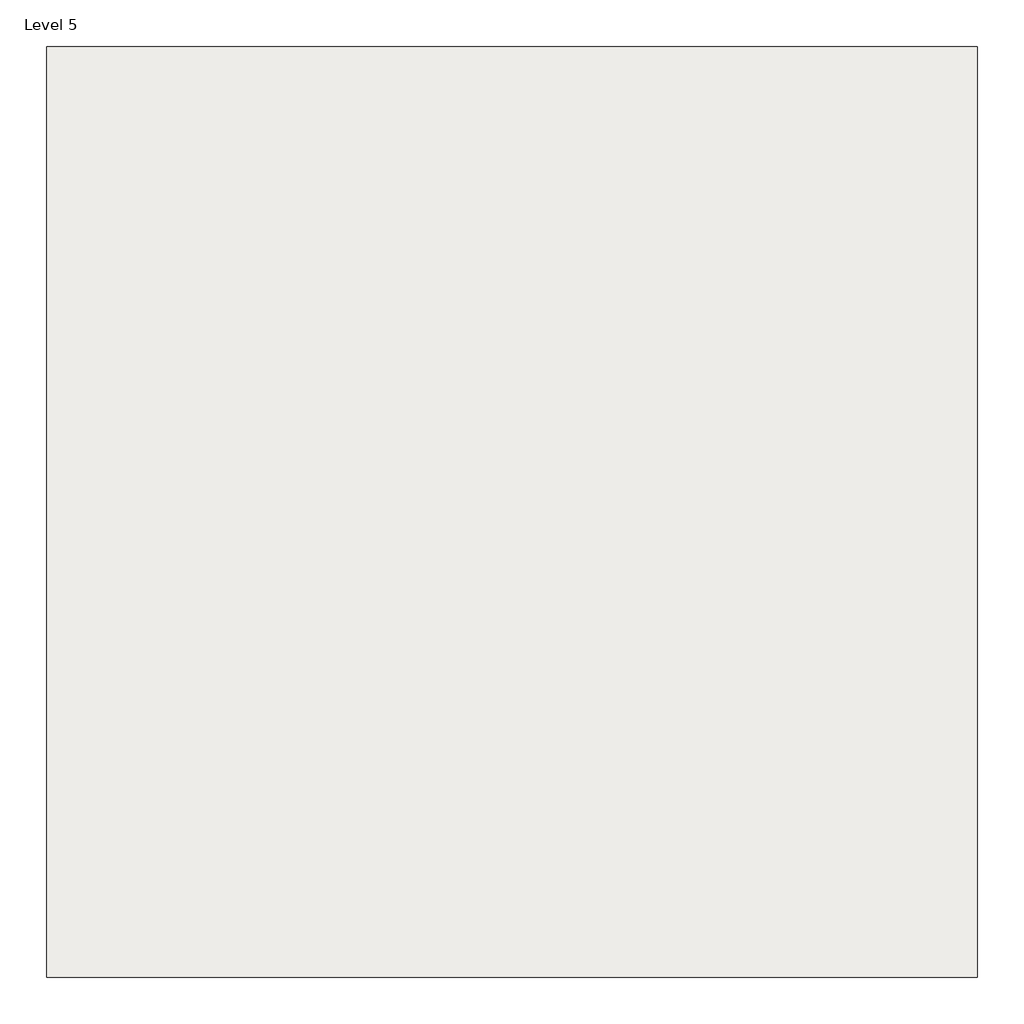
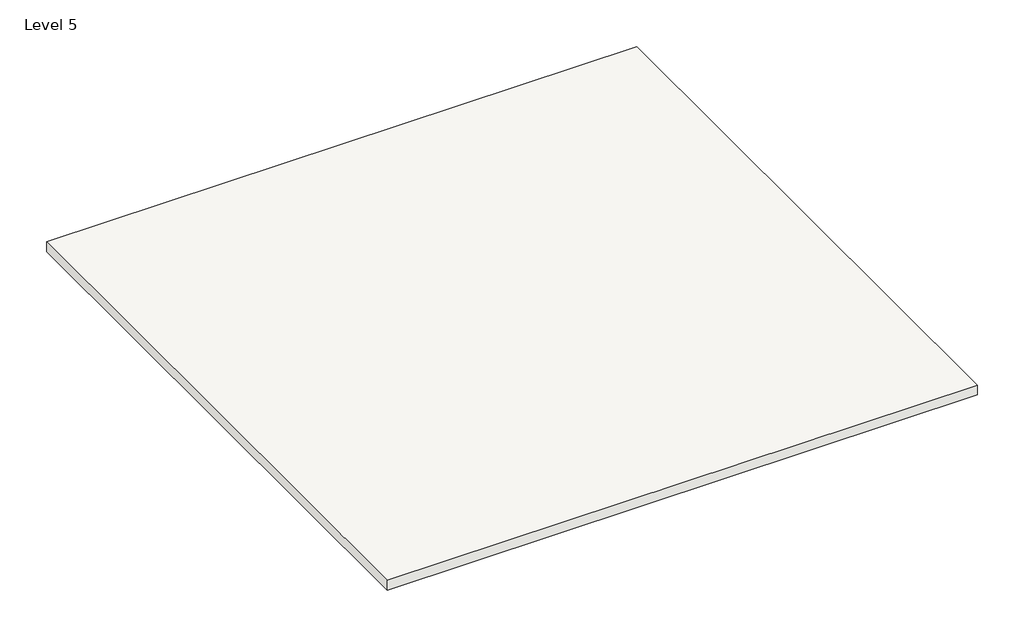
# One storey, incomplete: 1 roof.
"""IFC4 building model written with IfcOpenShell, lengths in millimetres."""

from ifc_helpers import new_model, si_unit, frame, origin, place, context, project, spatial, polyline, outline, extrude, element, save

model = new_model("IFC4")

# Units and contexts
model_context = context("Model", 3, world=origin())
ifc_project = project(units=[si_unit("LENGTHUNIT", "METRE", prefix="MILLI")], contexts=[model_context])

# Site, building, storey
site = spatial("IfcSite", under=ifc_project)
building = spatial("IfcBuilding", under=site)
storey = spatial("IfcBuildingStorey", under=building, Name="Level 5", Elevation=12192.0)

# Roof
placement = place(None, origin())
element("IfcRoof", 1, ObjectType="Generic - 12\"", at=placement, inside=storey, context=model_context, shape_type="SweptSolid", body=[
    extrude(outline(polyline([(406.4, 14579.6), (9245.6, 14579.6), (9245.6, 5740.4), (406.4, 5740.4), (406.4, 14579.6)])), frame((0.0, 0.0, 12192.0), z_axis=(0.0, 0.0, 1.0), x_axis=(1.0, 0.0, 0.0)), (0.0, 0.0, 1.0), 152.4),
])

save(model, "model.ifc")

# Revit data of these elements
# Type "Generic - 12\""
#   Assembly Code = "B1020"
#   Layers, outside or top first: 0' - 6" no material (function 1)
# Element 1 (IfcRoof, "Generic - 12\"")
#   built-in parameter 1001705 = 40.5 (stored number, unit not read)
#   built-in parameter 1001710 = 33615
#   Phase Created = New Construction
#   Materials on its faces: "Textile - Linen, Smooth", "Default Roof", "Clad - White"
# Materials
#   "Textile - Linen, Smooth": colour RGB 249 239 230, transparency 0
#   "Default Roof": colour RGB 88 101 114, transparency 0, Cost = 0
#   "Clad - White": class "Wood", colour RGB 242 242 238, transparency 0, Cost = 0
